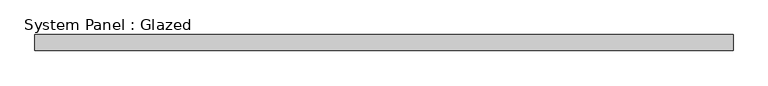
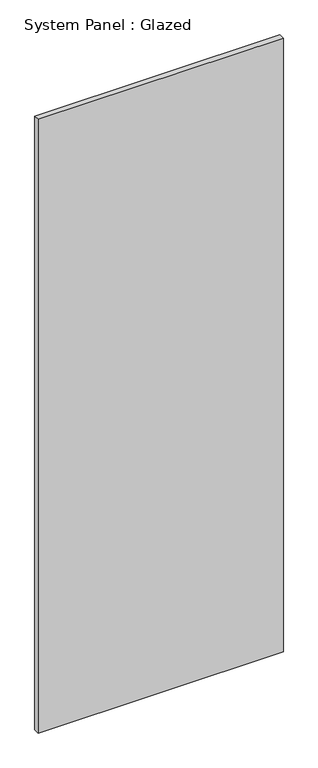
"""IFC4 building model written with IfcOpenShell, lengths in millimetres: plate geometry, System Panel : Glazed."""

from ifc_helpers import new_model, si_unit, origin, origin_with_axes, place, context, project, spatial, polyline, outline, extrude, source, transform, mapped, element, save


def system_panel_glazed_90a2254b(model_context):
    return source(origin(), model_context, "Body", "SweptSolid", [
        extrude(outline(polyline([(552.45, 19.05), (-552.45, 19.05), (-552.45, 44.45), (552.45, 44.45), (552.45, 19.05)])), origin_with_axes(), (0.0, 0.0, 1.0), 2921.0),
    ])


if __name__ == "__main__":
    model = new_model("IFC4")
    model_context = context("Model", 3, world=origin())
    ifc_project = project(units=[si_unit("LENGTHUNIT", "METRE", prefix="MILLI")], contexts=[model_context])
    site = spatial("IfcSite", under=ifc_project)
    building = spatial("IfcBuilding", under=site)
    placement = place(None, origin())
    system_panel_glazed_shape = system_panel_glazed_90a2254b(model_context)
    element("IfcPlate", 1, ObjectType="System Panel : Glazed", at=placement, inside=building, context=model_context, shape_type="MappedRepresentation", body=[
        mapped(system_panel_glazed_shape, transform((0.0, 0.0, 0.0), x_axis=(1.0, 0.0, 0.0), y_axis=(0.0, 1.0, 0.0), z_axis=(0.0, 0.0, 1.0))),
    ])
    save(model, "model.ifc")

# Revit data of these elements
# Type "System Panel : Glazed"
#   Construction Type Id = "GSP4R"
#   Analytic Construction = "1/8 in Pilkington single glazing"
#   Visual Light Transmittance = 0.9
#   Solar Heat Gain Coefficient = 0.86
#   Heat Transfer Coefficient (U) = 1.18115 BTU/(h·ft²·°F)
# Element 1 (IfcPlate, "System Panel : Glazed")
#   Materials on its faces: "Glass"
# Materials
#   "Glass": class "Glass", colour RGB 0 128 192, transparency 0.75, Description = "Soda Lime Glass", Cost = 0
